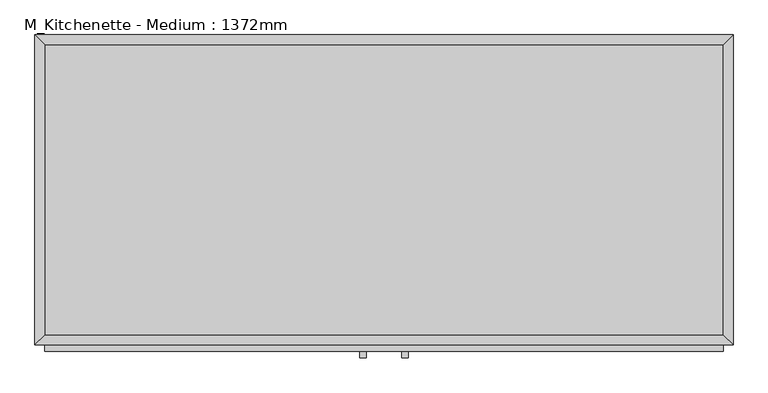
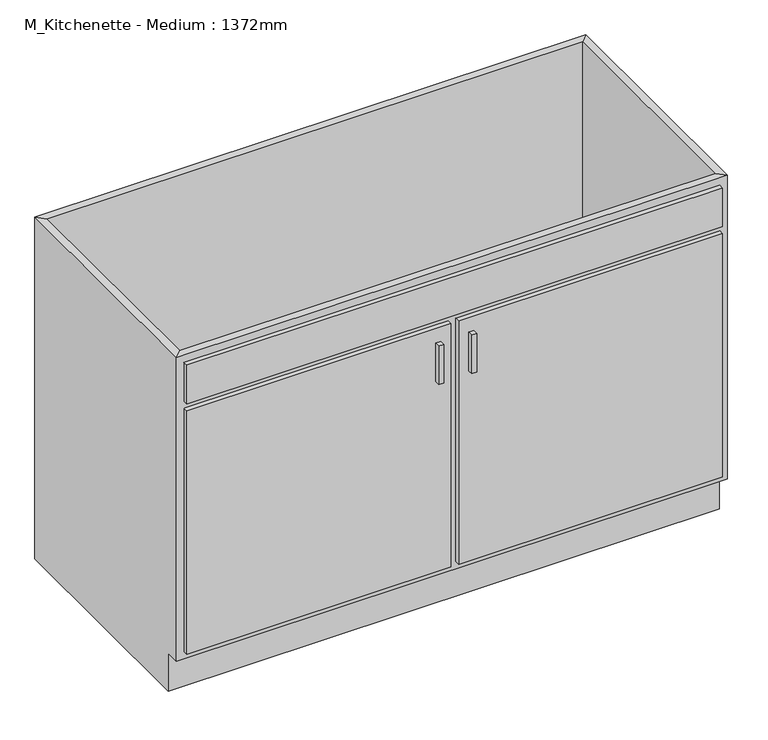
"""IFC4 building model written with IfcOpenShell, lengths in millimetres: proxy geometry, M_Kitchenette - Medium : 1372mm."""

from ifc_helpers import new_model, si_unit, frame, origin, place, context, project, spatial, polyline, outline, extrude, faceted_brep, source, transform, mapped, element, save


def m_kitchenette_medium_1372mm_e05c6bec(model_context):
    return source(origin(), model_context, "Body", "SolidModel", [
        faceted_brep([(685.6877049, -590.95, 900.0), (685.6877049, -590.95, 100.0), (-648.2122951, -590.95, 100.0), (-648.2122951, -590.95, 900.0), (-667.2622951, -610.0, 900.0), (704.7377049, -610.0, 900.0), (-667.2622951, -610.0, 100.0), (704.7377049, -610.0, 100.0), (-648.2122951, -575.0, 100.0), (-648.2122951, -19.05, 100.0), (-648.2122951, -19.05, 900.0), (-667.2622951, 0.0, 900.0), (-667.2622951, 0.0, 0.0), (-667.2622951, -575.0, 0.0), (-667.2622951, -575.0, 100.0), (685.6877049, -19.05, 100.0), (685.6877049, -19.05, 900.0), (704.7377049, 0.0, 900.0), (704.7377049, 0.0, 0.0), (685.6877049, -575.0, 100.0), (704.7377049, -575.0, 100.0), (704.7377049, -575.0, 0.0)], [[[0, 1, 2, 3]], [[0, 3, 4, 5]], [[5, 4, 6, 7]], [[2, 1, 7, 6]], [[3, 2, 8, 9, 10]], [[4, 3, 10, 11]], [[6, 4, 11, 12, 13, 14]], [[2, 6, 14, 8]], [[10, 9, 15, 16]], [[11, 10, 16, 17]], [[12, 11, 17, 18]], [[1, 0, 16, 15, 19]], [[0, 5, 17, 16]], [[5, 7, 20, 21, 18, 17]], [[7, 1, 19, 20]], [[8, 19, 15, 9]], [[18, 21, 13, 12]], [[13, 21, 20, 19, 8, 14]]]),
        extrude(outline(polyline([(-16.1872951, -635.4), (-28.8872951, -635.4), (-28.8872951, -622.7), (-16.1872951, -622.7), (-16.1872951, -635.4)])), frame((0.0, 0.0, 620.6), z_axis=(0.0, 0.0, 1.0), x_axis=(1.0, 0.0, 0.0)), (0.0, 0.0, 1.0), 101.6),
        extrude(outline(polyline([(66.3627049, -635.4), (53.6627049, -635.4), (53.6627049, -622.7), (66.3627049, -622.7), (66.3627049, -635.4)])), frame((0.0, 0.0, 620.6), z_axis=(0.0, 0.0, 1.0), x_axis=(1.0, 0.0, 0.0)), (0.0, 0.0, 1.0), 101.6),
        extrude(outline(polyline([(685.6877049, -19.05), (685.6877049, -590.95), (-648.2122951, -590.95), (-648.2122951, -19.05), (685.6877049, -19.05)])), frame((0.0, 0.0, 100.0), z_axis=(0.0, 0.0, 1.0), x_axis=(1.0, 0.0, 0.0)), (0.0, 0.0, 1.0), 19.05),
        extrude(outline(polyline([(9.2127049, -622.7), (-648.2122951, -622.7), (-648.2122951, -610.0), (9.2127049, -610.0), (9.2127049, -622.7)])), frame((0.0, 0.0, 119.05), z_axis=(0.0, 0.0, 1.0), x_axis=(1.0, 0.0, 0.0)), (0.0, 0.0, 1.0), 641.25),
        extrude(outline(polyline([(685.6877049, -622.7), (28.2627049, -622.7), (28.2627049, -610.0), (685.6877049, -610.0), (685.6877049, -622.7)])), frame((0.0, 0.0, 119.05), z_axis=(0.0, 0.0, 1.0), x_axis=(1.0, 0.0, 0.0)), (0.0, 0.0, 1.0), 641.25),
        extrude(outline(polyline([(685.6877049, -622.7), (-648.2122951, -622.7), (-648.2122951, -610.0), (685.6877049, -610.0), (685.6877049, -622.7)])), frame((0.0, 0.0, 779.35), z_axis=(0.0, 0.0, 1.0), x_axis=(1.0, 0.0, 0.0)), (0.0, 0.0, 1.0), 101.6),
    ])


if __name__ == "__main__":
    model = new_model("IFC4")
    model_context = context("Model", 3, world=origin())
    ifc_project = project(units=[si_unit("LENGTHUNIT", "METRE", prefix="MILLI")], contexts=[model_context])
    site = spatial("IfcSite", under=ifc_project)
    building = spatial("IfcBuilding", under=site)
    placement = place(None, origin())
    m_kitchenette_medium_1372mm_shape = m_kitchenette_medium_1372mm_e05c6bec(model_context)
    element("IfcBuildingElementProxy", 1, Name="M_Kitchenette - Medium : 1372mm", ObjectType="M_Kitchenette - Medium : 1372mm", at=placement, inside=building, context=model_context, shape_type="MappedRepresentation", body=[
        mapped(m_kitchenette_medium_1372mm_shape, transform((0.0, 0.0, 0.0), x_axis=(1.0, 0.0, 0.0), y_axis=(0.0, 1.0, 0.0), z_axis=(0.0, 0.0, 1.0))),
    ])
    save(model, "model.ifc")

# Revit data of these elements
# Type "M_Kitchenette - Medium : 1372mm"
#   Counter Length = 1980 mm
#   Cabinet Width = 1372 mm
#   Cabinet Height = 900 mm
#   Cabinet Depth = 610 mm
#   Toe Depth = 35 mm
#   Toe Height = 100 mm
#   Cabinet Material = Cabinets
#   Door/Drawer Material = Cabinets
#   Handle Material = Cabinets - Handles
#   Default Elevation = 0
# Element 1 (IfcBuildingElementProxy, "M_Kitchenette - Medium : 1372mm")
#   Materials on its faces: "Cabinets", "Cabinets - Handles"
# Materials
#   "Cabinets": colour RGB 249 249 249, transparency 0
#   "Cabinets - Handles": class "Metal", colour RGB 57 57 57, transparency 0
